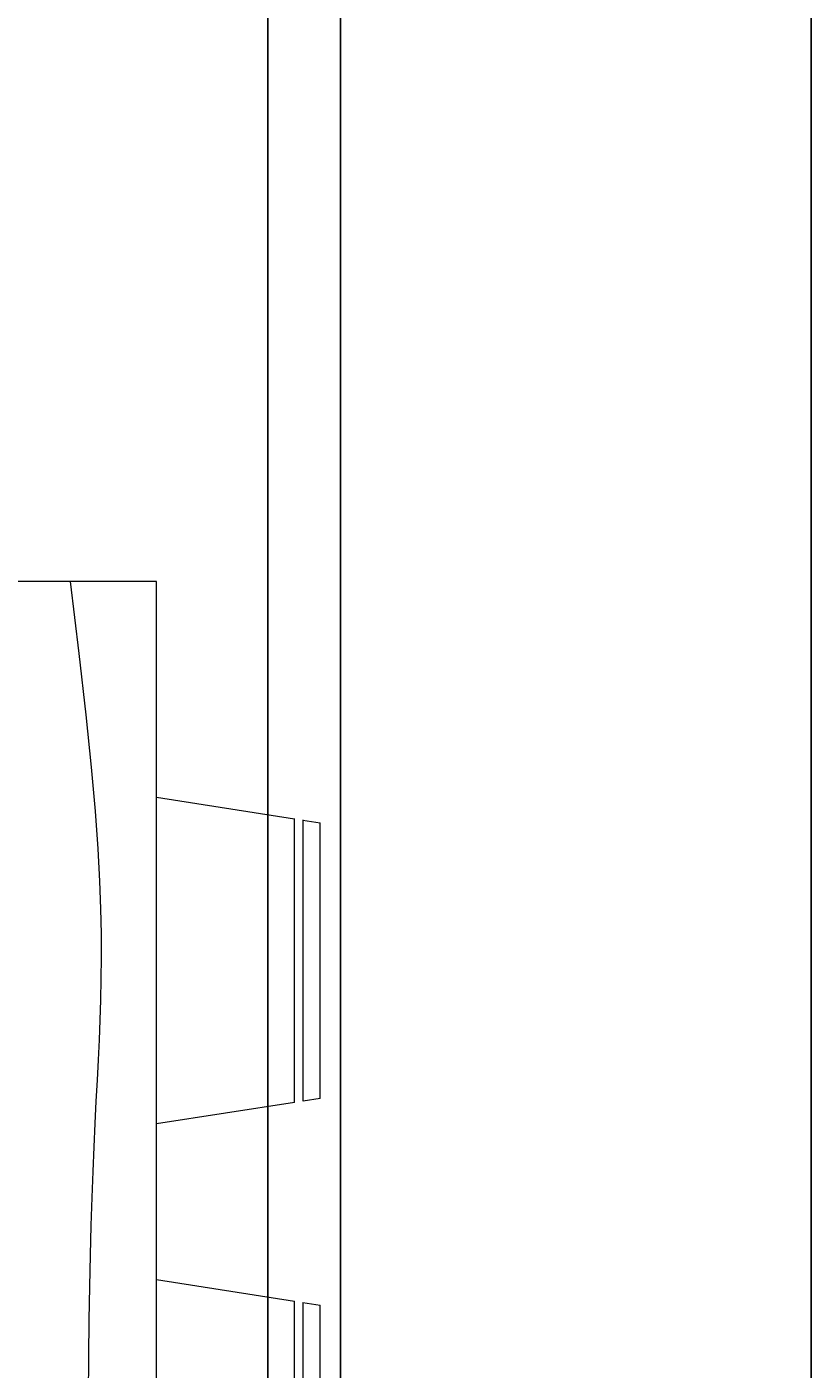
# Model space of a CAD drawing. Units: feet. Extents: x 1654 to 2985, y 1348 to 2230.
# Tile 31 of 53: x 2002 to 2042, y 1820 to 1889. Entities that reach past the tile are written whole.
import ezdxf

# ---------------------------------------------------------------- set-up
doc = ezdxf.new("R2010")
doc.units = ezdxf.units.FT
doc.layers.add('A-ANNO-DIMS', color=2, linetype='Continuous', lineweight=18)
doc.layers.add('A-FURN', color=8, linetype='Continuous', lineweight=13)
doc.styles.get("Standard").update_dxf_attribs({"font": 'arial.ttf'})
doc.dimstyles.get("Standard").update_dxf_attribs({"dimtxt": 0.18, "dimasz": 0.18, "dimexe": 0.18, "dimexo": 0.0625, "dimgap": 0.09, "dimtad": 0, "dimtih": 1, "dimtoh": 1, "dimdec": 4, "dimzin": 0, "dimdsep": 46, "dimtxsty": 'Standard', "dimcen": 0.09, "dimadec": 0, "dimazin": 0, "dimtfac": 1, "dimtdec": 4, "dimtofl": 0, "dimtmove": 0, "dimatfit": 3, "dimfxl": 1, "dimtolj": 1, "dimtzin": 0, "dimarcsym": 0})

# ---------------------------------------------------------------- blocks, each defined once
blk = doc.blocks.new('Dining Set - 36 x 72 in.')
for p, q in [((36, -18), (36, 18)), ((-36, -18), (36, -18)), ((-4.5152, -17.99762), (-5.7655, -25.99928)), ((5.7657, -26.0006), (4.5153, -17.99762)), ((23.4848, -17.99762), (22.2345, -25.99928)), ((-22.2304, -26), (-5.7608, -26)), ((5.7696, -26), (22.2392, -26)), ((-5.8416, -26.5), (-22.1534, -26.5)), ((-5.8437, -26.49967), (-6, -27.5)), ((6, -27.5), (5.8438, -26.50044)), ((22.1584, -26.5), (5.8466, -26.5)), ((22.1563, -26.49967), (22, -27.5)), ((-22, -27.5), (-6, -27.5)), ((6, -27.5), (22, -27.5))]:
    blk.add_line(p, q)
blk.add_lwpolyline([(-11.3027, -14.04297), (-8.9724, -14.05681), (-6.875, -14.08334), (-4.9224, -14.11833), (-3.0905, -14.16016), (-1.3709, -14.20785), (0.2448, -14.26042), (1.7647, -14.3169), (3.1973, -14.3763), (4.5507, -14.43767), (5.8333, -14.5), (7.0554, -14.5621), (8.235, -14.62175), (9.3922, -14.67652), (10.5469, -14.72396), (11.7192, -14.76164), (12.929, -14.78711), (14.1965, -14.79794), (15.5417, -14.79167), (16.9933, -14.76424), (18.6152, -14.70508), (20.4804, -14.60197), (22.6615, -14.44271), (25.2312, -14.21509), (28.2624, -13.9069), (31.8277, -13.50594), (36, -13)])
blk = doc.blocks.new('*D88')
at = {"layer": 'A-ANNO-DIMS', "color": 0, "lineweight": -2, "transparency": 16777216}
for p, q in [((2017.769, 1661.317), (2017.769, 2148.435)), ((2042.08, 1661.317), (2042.08, 2148.435)), ((2017.949, 2148.255), (2029.547, 2148.255)), ((2041.9, 2148.255), (2030.302, 2148.255))]:
    blk.add_line(p, q, dxfattribs=at)
at = {"layer": 'A-ANNO-DIMS', "color": 0, "transparency": 16777216}
for points in [[(2017.949, 2148.285), (2017.949, 2148.225), (2017.769, 2148.255)], [(2041.9, 2148.285), (2041.9, 2148.225), (2042.08, 2148.255)]]:
    blk.add_solid(points, dxfattribs=at)
at = {"layer": 'Defpoints', "color": 0, "transparency": 16777216}
for p in [(2017.769, 2148.255), (2017.769, 1661.255), (2042.08, 1661.255)]:
    blk.add_point(p, dxfattribs=at)
at = {"layer": 'A-ANNO-DIMS', "color": 0, "transparency": 16777216, "insert": (2029.925, 2148.255), "char_height": 0.18, "attachment_point": 5}
blk.add_mtext('\\A1;24.31', dxfattribs=at)
blk = doc.blocks.new('*D101')
at = {"layer": 'A-ANNO-DIMS', "color": 0, "lineweight": -2, "transparency": 16777216}
for p, q in [((1996.092, 2039.192), (1996.092, 1534.075)), ((2014.016, 2039.192), (2014.016, 1534.075)), ((1996.272, 1534.255), (2004.599, 1534.255)), ((2013.836, 1534.255), (2005.509, 1534.255))]:
    blk.add_line(p, q, dxfattribs=at)
at = {"layer": 'A-ANNO-DIMS', "color": 0, "transparency": 16777216}
for points in [[(1996.272, 1534.285), (1996.272, 1534.225), (1996.092, 1534.255)], [(2013.836, 1534.285), (2013.836, 1534.225), (2014.016, 1534.255)]]:
    blk.add_solid(points, dxfattribs=at)
at = {"layer": 'Defpoints', "color": 0, "transparency": 16777216}
for p in [(1996.092, 2039.255), (2014.016, 2039.255), (2014.016, 1534.255)]:
    blk.add_point(p, dxfattribs=at)
at = {"layer": 'A-ANNO-DIMS', "color": 0, "transparency": 16777216, "insert": (2005.054, 1534.255), "char_height": 0.18, "attachment_point": 5}
blk.add_mtext('\\A1;17.924', dxfattribs=at)

msp = doc.modelspace()

# ---------------------------------------------------------------- block references
at = {"layer": 'A-FURN', "xscale": 0.8893748792417884, "yscale": 0.8893748792417884, "zscale": 0.8893748792417884, "rotation": 90}
msp.add_blockref('Dining Set - 36 x 72 in.', (1992.2681, 1828.3522), dxfattribs=at)

# ---------------------------------------------------------------- dimensions: what is measured, and where the dimension line sits
at = {"layer": 'A-ANNO-DIMS'}
for base, p1, p2, override, picture, middle in [((2017.7694, 2148.2549), (2042.0798, 1661.2549), (2017.7694, 1661.2549), {"dimdec": 2, "dimlfac": 1, "dimrnd": 0, "dimzin": 0, "dimdsep": 46, "dimlunit": 2}, '*D88', (2029.9246, 2148.2549)), ((2014.016, 1534.2549), (1996.0924, 2039.2549), (2014.016, 2039.2549), {"dimdec": 3, "dimlfac": 1, "dimrnd": 0, "dimzin": 0, "dimdsep": 46, "dimlunit": 2}, '*D101', (2005.0542, 1534.2549))]:
    dim = msp.add_linear_dim(base=base, p1=p1, p2=p2, dimstyle='Standard', override=override, dxfattribs=at)
    dim.commit()
    dim.dimension.update_dxf_attribs({"geometry": picture, "text_midpoint": middle})

doc.saveas('drawing.dxf')
